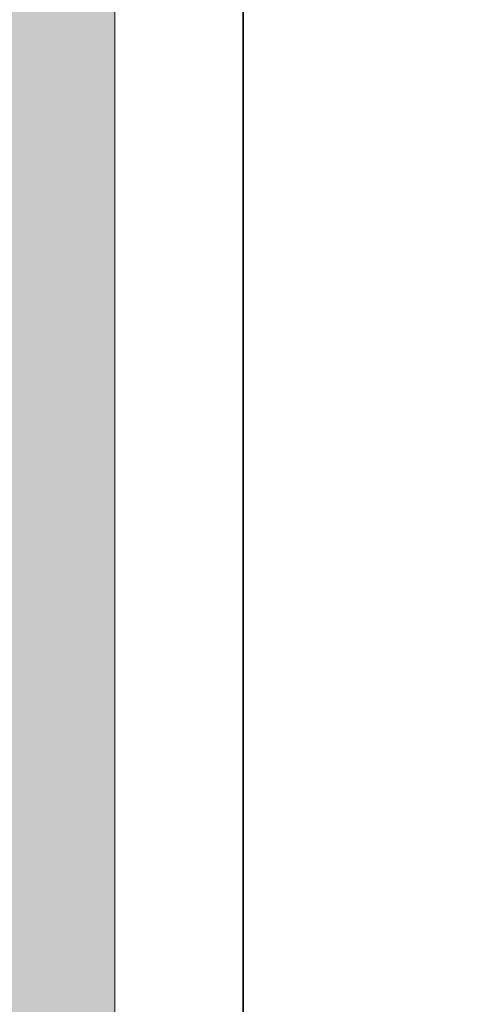
# Model space of a CAD drawing. Units: inches. Extents: x 1704 to 6393, y -157 to 1172.
# Tile 110 of 122: x 2716 to 2730, y 972 to 1003. Entities that reach past the tile are written whole.
import ezdxf

# ---------------------------------------------------------------- set-up
doc = ezdxf.new("R2010")
doc.units = ezdxf.units.IN
doc.header["$MEASUREMENT"] = 0
for name, color, linetype, lineweight in [('A-ANNO-DIMS', 7, 'Continuous', 13), ('C-PROP', 7, 'Continuous', 35), ('L-HRDS', 8, 'Continuous', 18)]:
    doc.layers.add(name, color=color, linetype=linetype, lineweight=lineweight)
doc.layers.add('L-HRDS-PATT', color=9, linetype='Continuous', lineweight=13, true_color=0xc5c1ba)
doc.styles.get("Standard").update_dxf_attribs({"font": 'arial.ttf'})
doc.dimstyles.get("Standard").update_dxf_attribs({"dimtxt": 6, "dimasz": 2, "dimexe": 0.18, "dimexo": 0.0625, "dimgap": 0.09, "dimtad": 0, "dimtih": 1, "dimtoh": 1, "dimdec": 1, "dimzin": 0, "dimdsep": 46, "dimlunit": 3, "dimtxsty": 'Standard', "dimblk": 'ARCHTICK', "dimcen": 0.09, "dimadec": 0, "dimazin": 0, "dimtfac": 1, "dimtdec": 1, "dimtofl": 0, "dimtmove": 0, "dimatfit": 3, "dimfxl": 1, "dimtolj": 1, "dimtzin": 0, "dimarcsym": 0})

# ---------------------------------------------------------------- blocks, each defined once
blk = doc.blocks.new('_ArchTick')
at = {"color": 0, "linetype": 'ByBlock', "const_width": 0.15}
blk.add_lwpolyline([(-0.5, -0.5), (0.5, 0.5)], dxfattribs=at)
blk = doc.blocks.new('*D91')
at = {"layer": 'A-ANNO-DIMS', "color": 0, "lineweight": -2, "transparency": 16777216}
for p, q in [((2723.411, 1033.213), (2784.529, 1033.213)), ((2784.349, 1033.213), (2784.349, 517.868)), ((2784.349, -3.787), (2784.349, 511.557)), ((2723.411, -3.787), (2784.529, -3.787))]:
    blk.add_line(p, q, dxfattribs=at)
at = {"layer": 'Defpoints', "color": 0, "lineweight": -3, "transparency": 16777216}
for p in [(2723.349, 1033.213), (2784.349, 1033.213), (2723.349, -3.787)]:
    blk.add_point(p, dxfattribs=at)
at = {"layer": 'A-ANNO-DIMS', "color": 0, "lineweight": -2, "transparency": 16777216, "xscale": 2, "yscale": 2, "zscale": 2}
for p, rotation in [((2784.349, 1033.213), 90), ((2784.349, -3.787), 270)]:
    blk.add_blockref('_ArchTick', p, dxfattribs=dict(at, rotation=rotation))
at = {"layer": 'A-ANNO-DIMS', "color": 0, "transparency": 16777216, "insert": (2784.349, 514.713), "char_height": 6, "attachment_point": 5}
blk.add_mtext('\\A1;1037', dxfattribs=at)
blk = doc.blocks.new('*D95')
at = {"layer": 'A-ANNO-DIMS', "color": 0, "lineweight": -2, "transparency": 16777216}
for p, q in [((2605.349, 895.275), (2605.349, 1105.287)), ((2723.349, 895.275), (2723.349, 1105.287)), ((2605.349, 1105.107), (2657.907, 1105.107)), ((2723.349, 1105.107), (2670.791, 1105.107))]:
    blk.add_line(p, q, dxfattribs=at)
at = {"layer": 'Defpoints', "color": 0, "lineweight": -3, "transparency": 16777216}
for p in [(2723.349, 1105.107), (2605.349, 895.213), (2723.349, 895.213)]:
    blk.add_point(p, dxfattribs=at)
at = {"layer": 'A-ANNO-DIMS', "color": 0, "lineweight": -2, "transparency": 16777216, "xscale": 2, "yscale": 2, "zscale": 2, "rotation": 180}
blk.add_blockref('_ArchTick', (2605.349, 1105.107), dxfattribs=at)
at = {"layer": 'A-ANNO-DIMS', "color": 0, "lineweight": -2, "transparency": 16777216, "xscale": 2, "yscale": 2, "zscale": 2}
blk.add_blockref('_ArchTick', (2723.349, 1105.107), dxfattribs=at)
at = {"layer": 'A-ANNO-DIMS', "color": 0, "transparency": 16777216, "insert": (2664.349, 1105.107), "char_height": 6, "attachment_point": 5}
blk.add_mtext('\\A1;118', dxfattribs=at)

msp = doc.modelspace()

# ---------------------------------------------------------------- hatches: boundary and pattern name
at = {"layer": 'L-HRDS-PATT', "transparency": 33554661}
h = msp.add_hatch(color=256, dxfattribs=at)
h.dxf.hatch_style = 1
h.paths.add_polyline_path([(2719.349, 1033.213), (2664.349, 1033.213), (2664.349, 895.213), (2719.349, 895.213)])
h.paths.add_polyline_path([(2719.349, 895.213), (2664.349, 895.213), (2605.349, 895.213), (2605.349, 872.213), (2719.349, 872.213)])
h.paths.add_polyline_path([(2719.349, 872.213), (2605.349, 872.213), (2605.349, 854.213), (2601.349, 854.213, -0.121066), (2618.034, 850.113), (2618.05, 850.14), (2619.349, 849.39), (2601.349, 818.213), (2605.349, 818.213), (2605.349, 794.213), (2605.349, 754.213), (2631.349, 754.213), (2631.349, 716.213), (2719.349, 716.213)])

# ---------------------------------------------------------------- linework, layer by layer
at = {"layer": 'C-PROP'}
msp.add_line((2723.349, -3.787), (2723.349, 1033.213), dxfattribs=at)
at = {"layer": 'L-HRDS'}
msp.add_line((2719.349, 5.658), (2719.349, 1033.213), dxfattribs=at)

# ---------------------------------------------------------------- dimensions: what is measured, and where the dimension line sits
at = {"layer": 'A-ANNO-DIMS'}
dim = msp.add_linear_dim(base=(2723.349, 1105.107), p1=(2605.349, 895.213), p2=(2723.349, 895.213), dimstyle='Standard', override={"dimdec": 0, "dimlfac": 1, "dimrnd": 0, "dimzin": 0, "dimdsep": 46, "dimlunit": 2}, dxfattribs=at)
dim.commit()
dim.dimension.update_dxf_attribs({"geometry": '*D95', "text_midpoint": (2664.349, 1105.107)})
dim = msp.add_linear_dim(base=(2784.349, 1033.213), p1=(2723.349, -3.787), p2=(2723.349, 1033.213), angle=90, dimstyle='Standard', override={"dimdec": 0, "dimlfac": 1, "dimrnd": 0, "dimzin": 0, "dimdsep": 46, "dimlunit": 2}, dxfattribs=at)
dim.commit()
dim.dimension.update_dxf_attribs({"geometry": '*D91', "text_midpoint": (2784.349, 514.713)})

doc.saveas('drawing.dxf')
